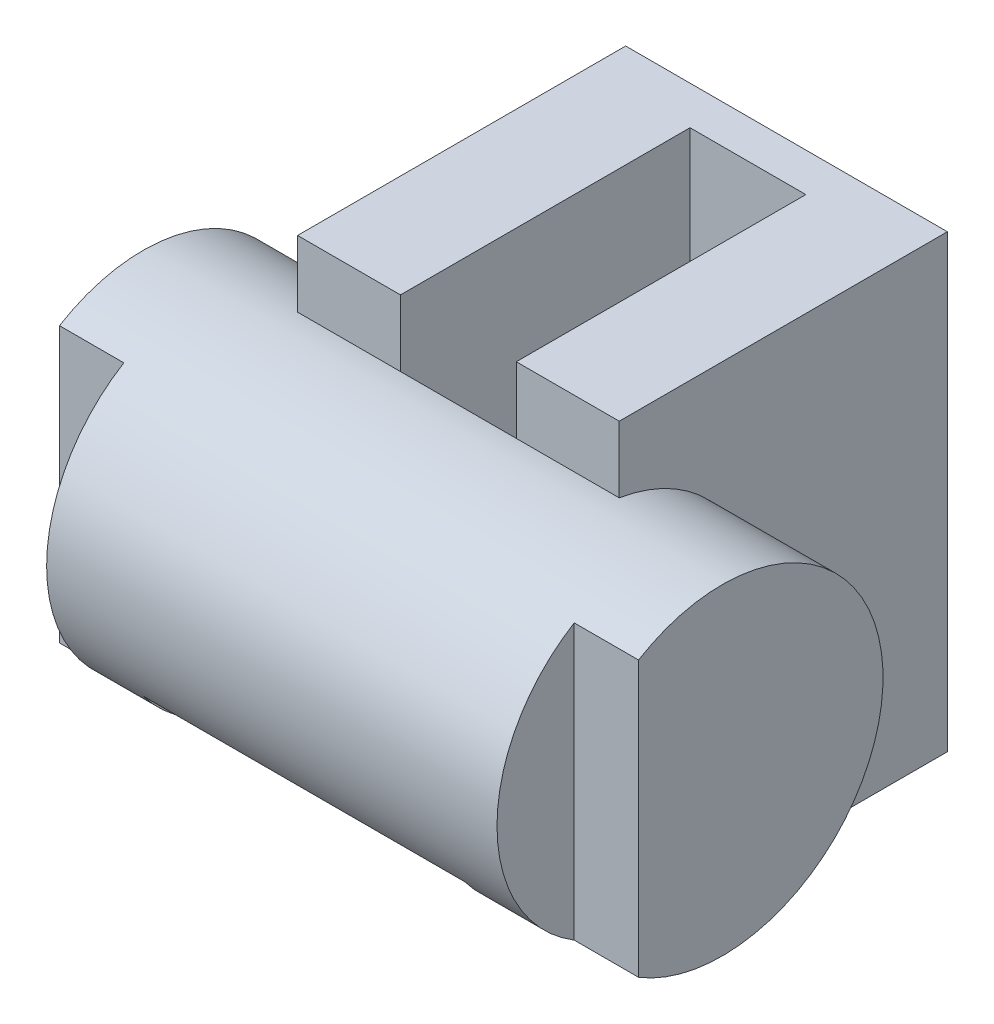
ISO-10303-21;
HEADER;
FILE_DESCRIPTION(('STEP AP214'),'2;1');
FILE_NAME('part.step','',(''),(''),'','','');
FILE_SCHEMA(('AUTOMOTIVE_DESIGN { 1 0 10303 214 1 1 1 1 }'));
ENDSEC;
DATA;
#1=APPLICATION_CONTEXT('core data for automotive mechanical design processes');
#2=APPLICATION_PROTOCOL_DEFINITION('international standard','automotive_design',2000,#1);
#3=PRODUCT_CONTEXT('',#1,'mechanical');
#4=PRODUCT('Part','Part','',(#3));
#5=PRODUCT_RELATED_PRODUCT_CATEGORY('part','',(#4));
#6=PRODUCT_DEFINITION_FORMATION('','',#4);
#7=PRODUCT_DEFINITION_CONTEXT('part definition',#1,'design');
#8=PRODUCT_DEFINITION('design','',#6,#7);
#9=PRODUCT_DEFINITION_SHAPE('','',#8);
#10=(LENGTH_UNIT() NAMED_UNIT(*) SI_UNIT(.MILLI.,.METRE.));
#11=(NAMED_UNIT(*) PLANE_ANGLE_UNIT() SI_UNIT($,.RADIAN.));
#12=(NAMED_UNIT(*) SI_UNIT($,.STERADIAN.) SOLID_ANGLE_UNIT());
#13=UNCERTAINTY_MEASURE_WITH_UNIT(LENGTH_MEASURE(1.E-05),#10,'distance_accuracy_value','');
#14=(GEOMETRIC_REPRESENTATION_CONTEXT(3) GLOBAL_UNCERTAINTY_ASSIGNED_CONTEXT((#13)) GLOBAL_UNIT_ASSIGNED_CONTEXT((#10,
#11,#12)) REPRESENTATION_CONTEXT('',''));
#15=CARTESIAN_POINT('',(0.,0.,0.));
#16=DIRECTION('',(0.,0.,1.));
#17=DIRECTION('',(1.,0.,0.));
#18=AXIS2_PLACEMENT_3D('',#15,#16,#17);
#19=CARTESIAN_POINT('',(70.,-35.,58.));
#20=DIRECTION('',(-1.,0.,0.));
#21=DIRECTION('',(0.,0.,1.));
#22=AXIS2_PLACEMENT_3D('',#19,#20,#21);
#23=CYLINDRICAL_SURFACE('',#22,25.);
#24=DIRECTION('',(-1.,0.,0.));
#25=VECTOR('',#24,1.);
#26=CARTESIAN_POINT('',(70.,-10.3220746414939,54.));
#27=LINE('',#26,#25);
#28=CARTESIAN_POINT('',(16.,-10.3220746414939,54.));
#29=VERTEX_POINT('',#28);
#30=CARTESIAN_POINT('',(34.,-10.3220746414939,54.));
#31=VERTEX_POINT('',#30);
#32=EDGE_CURVE('E214',#29,#31,#27,.F.);
#33=ORIENTED_EDGE('',*,*,#32,.F.);
#34=DIRECTION('',(-1.,0.,0.));
#35=VECTOR('',#34,1.);
#36=CARTESIAN_POINT('',(70.,-10.3220746414939,54.));
#37=LINE('',#36,#35);
#38=CARTESIAN_POINT('',(0.,-10.3220746414939,54.));
#39=VERTEX_POINT('',#38);
#40=EDGE_CURVE('E233',#29,#39,#37,.T.);
#41=ORIENTED_EDGE('',*,*,#40,.T.);
#42=CARTESIAN_POINT('',(0.,-35.,58.));
#43=DIRECTION('',(-1.,0.,0.));
#44=DIRECTION('',(0.,0.,1.));
#45=AXIS2_PLACEMENT_3D('',#42,#43,#44);
#46=CIRCLE('',#45,25.);
#47=CARTESIAN_POINT('',(0.,-50.,38.));
#48=VERTEX_POINT('',#47);
#49=EDGE_CURVE('E220',#39,#48,#46,.T.);
#50=ORIENTED_EDGE('',*,*,#49,.T.);
#51=CARTESIAN_POINT('',(0.,-35.,58.));
#52=DIRECTION('',(1.,0.,0.));
#53=DIRECTION('',(0.,0.,-1.));
#54=AXIS2_PLACEMENT_3D('',#51,#52,#53);
#55=CIRCLE('',#54,25.);
#56=CARTESIAN_POINT('',(0.,-50.,78.));
#57=VERTEX_POINT('',#56);
#58=EDGE_CURVE('E323',#48,#57,#55,.F.);
#59=ORIENTED_EDGE('',*,*,#58,.T.);
#60=DIRECTION('',(-1.,0.,0.));
#61=VECTOR('',#60,1.);
#62=CARTESIAN_POINT('',(70.,-50.,78.));
#63=LINE('',#62,#61);
#64=CARTESIAN_POINT('',(50.,-50.,78.));
#65=VERTEX_POINT('',#64);
#66=EDGE_CURVE('E52',#57,#65,#63,.F.);
#67=ORIENTED_EDGE('',*,*,#66,.T.);
#68=CARTESIAN_POINT('',(50.,-35.,58.));
#69=DIRECTION('',(-1.,0.,0.));
#70=DIRECTION('',(0.,0.,1.));
#71=AXIS2_PLACEMENT_3D('',#68,#69,#70);
#72=CIRCLE('',#71,25.);
#73=CARTESIAN_POINT('',(50.,-50.,38.));
#74=VERTEX_POINT('',#73);
#75=EDGE_CURVE('E11',#65,#74,#72,.F.);
#76=ORIENTED_EDGE('',*,*,#75,.T.);
#77=CARTESIAN_POINT('',(50.,-35.,58.));
#78=DIRECTION('',(-1.,0.,0.));
#79=DIRECTION('',(0.,0.,1.));
#80=AXIS2_PLACEMENT_3D('',#77,#78,#79);
#81=CIRCLE('',#80,25.);
#82=CARTESIAN_POINT('',(50.,-10.3220746414939,54.));
#83=VERTEX_POINT('',#82);
#84=EDGE_CURVE('E226',#83,#74,#81,.T.);
#85=ORIENTED_EDGE('',*,*,#84,.F.);
#86=DIRECTION('',(-1.,0.,0.));
#87=VECTOR('',#86,1.);
#88=CARTESIAN_POINT('',(70.,-10.3220746414939,54.));
#89=LINE('',#88,#87);
#90=EDGE_CURVE('E324',#83,#31,#89,.T.);
#91=ORIENTED_EDGE('',*,*,#90,.T.);
#92=EDGE_LOOP('',(#33,#41,#50,#59,#67,#76,#85,#91));
#93=FACE_BOUND('',#92,.T.);
#94=CARTESIAN_POINT('',(-20.,-35.,58.));
#95=DIRECTION('',(-1.,0.,0.));
#96=DIRECTION('',(0.,0.,1.));
#97=AXIS2_PLACEMENT_3D('',#94,#95,#96);
#98=CIRCLE('',#97,25.);
#99=CARTESIAN_POINT('',(-20.,-13.6458434959374,71.));
#100=VERTEX_POINT('',#99);
#101=CARTESIAN_POINT('',(-20.,-56.3541565040626,71.));
#102=VERTEX_POINT('',#101);
#103=EDGE_CURVE('E221',#100,#102,#98,.T.);
#104=ORIENTED_EDGE('',*,*,#103,.F.);
#105=DIRECTION('',(-1.,0.,0.));
#106=VECTOR('',#105,1.);
#107=CARTESIAN_POINT('',(-10.,-13.6458434959374,71.));
#108=LINE('',#107,#106);
#109=CARTESIAN_POINT('',(-10.,-13.6458434959374,71.));
#110=VERTEX_POINT('',#109);
#111=EDGE_CURVE('E69',#110,#100,#108,.T.);
#112=ORIENTED_EDGE('',*,*,#111,.F.);
#113=CARTESIAN_POINT('',(-10.,-35.,58.));
#114=DIRECTION('',(-1.,0.,0.));
#115=DIRECTION('',(0.,0.,1.));
#116=AXIS2_PLACEMENT_3D('',#113,#114,#115);
#117=CIRCLE('',#116,25.);
#118=CARTESIAN_POINT('',(-10.,-56.3541565040626,71.));
#119=VERTEX_POINT('',#118);
#120=EDGE_CURVE('E196',#119,#110,#117,.T.);
#121=ORIENTED_EDGE('',*,*,#120,.F.);
#122=DIRECTION('',(-1.,0.,0.));
#123=VECTOR('',#122,1.);
#124=CARTESIAN_POINT('',(-10.,-56.3541565040626,71.));
#125=LINE('',#124,#123);
#126=EDGE_CURVE('E198',#119,#102,#125,.T.);
#127=ORIENTED_EDGE('',*,*,#126,.T.);
#128=EDGE_LOOP('',(#104,#112,#121,#127));
#129=FACE_BOUND('',#128,.T.);
#130=CARTESIAN_POINT('',(60.,-35.,58.));
#131=DIRECTION('',(1.,0.,0.));
#132=DIRECTION('',(0.,0.,-1.));
#133=AXIS2_PLACEMENT_3D('',#130,#131,#132);
#134=CIRCLE('',#133,25.);
#135=CARTESIAN_POINT('',(60.,-13.6458434959373,71.));
#136=VERTEX_POINT('',#135);
#137=CARTESIAN_POINT('',(60.,-56.3541565040626,71.));
#138=VERTEX_POINT('',#137);
#139=EDGE_CURVE('E183',#136,#138,#134,.T.);
#140=ORIENTED_EDGE('',*,*,#139,.F.);
#141=DIRECTION('',(1.,0.,0.));
#142=VECTOR('',#141,1.);
#143=CARTESIAN_POINT('',(60.,-13.6458434959373,71.));
#144=LINE('',#143,#142);
#145=CARTESIAN_POINT('',(70.,-13.6458434959373,71.));
#146=VERTEX_POINT('',#145);
#147=EDGE_CURVE('E172',#136,#146,#144,.T.);
#148=ORIENTED_EDGE('',*,*,#147,.T.);
#149=CARTESIAN_POINT('',(70.,-35.,58.));
#150=DIRECTION('',(-1.,0.,0.));
#151=DIRECTION('',(0.,0.,1.));
#152=AXIS2_PLACEMENT_3D('',#149,#150,#151);
#153=CIRCLE('',#152,25.);
#154=CARTESIAN_POINT('',(70.,-56.3541565040626,71.));
#155=VERTEX_POINT('',#154);
#156=EDGE_CURVE('E223',#146,#155,#153,.T.);
#157=ORIENTED_EDGE('',*,*,#156,.T.);
#158=DIRECTION('',(1.,0.,0.));
#159=VECTOR('',#158,1.);
#160=CARTESIAN_POINT('',(60.,-56.3541565040626,71.));
#161=LINE('',#160,#159);
#162=EDGE_CURVE('E58',#138,#155,#161,.T.);
#163=ORIENTED_EDGE('',*,*,#162,.F.);
#164=EDGE_LOOP('',(#140,#148,#157,#163));
#165=FACE_BOUND('',#164,.T.);
#166=ADVANCED_FACE('F44',(#93,#129,#165),#23,.T.);
#167=CARTESIAN_POINT('',(70.,-35.,58.));
#168=DIRECTION('',(-1.,0.,0.));
#169=DIRECTION('',(0.,0.,1.));
#170=AXIS2_PLACEMENT_3D('',#167,#168,#169);
#171=PLANE('',#170);
#172=DIRECTION('',(0.,-1.,0.));
#173=VECTOR('',#172,1.);
#174=CARTESIAN_POINT('',(70.,0.,71.));
#175=LINE('',#174,#173);
#176=EDGE_CURVE('E177',#146,#155,#175,.T.);
#177=ORIENTED_EDGE('',*,*,#176,.T.);
#178=ORIENTED_EDGE('',*,*,#156,.F.);
#179=EDGE_LOOP('',(#177,#178));
#180=FACE_BOUND('',#179,.T.);
#181=ADVANCED_FACE('F356',(#180),#171,.F.);
#182=CARTESIAN_POINT('',(-20.,-35.,58.));
#183=DIRECTION('',(-1.,0.,0.));
#184=DIRECTION('',(0.,0.,1.));
#185=AXIS2_PLACEMENT_3D('',#182,#183,#184);
#186=PLANE('',#185);
#187=ORIENTED_EDGE('',*,*,#103,.T.);
#188=DIRECTION('',(0.,1.,0.));
#189=VECTOR('',#188,1.);
#190=CARTESIAN_POINT('',(-20.,0.,71.));
#191=LINE('',#190,#189);
#192=EDGE_CURVE('E191',#102,#100,#191,.T.);
#193=ORIENTED_EDGE('',*,*,#192,.T.);
#194=EDGE_LOOP('',(#187,#193));
#195=FACE_BOUND('',#194,.T.);
#196=ADVANCED_FACE('F361',(#195),#186,.T.);
#197=CARTESIAN_POINT('',(0.,0.,9.));
#198=DIRECTION('',(1.,0.,0.));
#199=DIRECTION('',(0.,0.,-1.));
#200=AXIS2_PLACEMENT_3D('',#197,#198,#199);
#201=PLANE('',#200);
#202=ORIENTED_EDGE('',*,*,#49,.F.);
#203=DIRECTION('',(0.,1.,0.));
#204=VECTOR('',#203,1.);
#205=CARTESIAN_POINT('',(0.,0.,54.));
#206=LINE('',#205,#204);
#207=CARTESIAN_POINT('',(0.,0.,54.));
#208=VERTEX_POINT('',#207);
#209=EDGE_CURVE('E281',#39,#208,#206,.T.);
#210=ORIENTED_EDGE('',*,*,#209,.T.);
#211=DIRECTION('',(0.,0.,-1.));
#212=VECTOR('',#211,1.);
#213=CARTESIAN_POINT('',(0.,0.,9.));
#214=LINE('',#213,#212);
#215=CARTESIAN_POINT('',(0.,0.,3.));
#216=VERTEX_POINT('',#215);
#217=EDGE_CURVE('E319',#208,#216,#214,.T.);
#218=ORIENTED_EDGE('',*,*,#217,.T.);
#219=DIRECTION('',(0.,1.,0.));
#220=VECTOR('',#219,1.);
#221=CARTESIAN_POINT('',(0.,0.,3.));
#222=LINE('',#221,#220);
#223=CARTESIAN_POINT('',(0.,-70.,3.));
#224=VERTEX_POINT('',#223);
#225=EDGE_CURVE('E257',#224,#216,#222,.T.);
#226=ORIENTED_EDGE('',*,*,#225,.F.);
#227=DIRECTION('',(0.,0.,-1.));
#228=VECTOR('',#227,1.);
#229=CARTESIAN_POINT('',(0.,-70.,9.));
#230=LINE('',#229,#228);
#231=CARTESIAN_POINT('',(0.,-70.,23.));
#232=VERTEX_POINT('',#231);
#233=EDGE_CURVE('E314',#232,#224,#230,.T.);
#234=ORIENTED_EDGE('',*,*,#233,.F.);
#235=DIRECTION('',(0.,-1.,0.));
#236=VECTOR('',#235,1.);
#237=CARTESIAN_POINT('',(0.,-70.,23.));
#238=LINE('',#237,#236);
#239=CARTESIAN_POINT('',(0.,-50.,23.));
#240=VERTEX_POINT('',#239);
#241=EDGE_CURVE('E246',#240,#232,#238,.T.);
#242=ORIENTED_EDGE('',*,*,#241,.F.);
#243=DIRECTION('',(0.,0.,1.));
#244=VECTOR('',#243,1.);
#245=CARTESIAN_POINT('',(0.,-50.,54.));
#246=LINE('',#245,#244);
#247=EDGE_CURVE('E276',#240,#48,#246,.T.);
#248=ORIENTED_EDGE('',*,*,#247,.T.);
#249=EDGE_LOOP('',(#202,#210,#218,#226,#234,#242,#248));
#250=FACE_BOUND('',#249,.T.);
#251=ADVANCED_FACE('F383',(#250),#201,.F.);
#252=CARTESIAN_POINT('',(16.,-50.,54.));
#253=DIRECTION('',(0.,-1.,0.));
#254=DIRECTION('',(0.,0.,-1.));
#255=AXIS2_PLACEMENT_3D('',#252,#253,#254);
#256=PLANE('',#255);
#257=DIRECTION('',(-1.,0.,0.));
#258=VECTOR('',#257,1.);
#259=CARTESIAN_POINT('',(16.,-50.,54.));
#260=LINE('',#259,#258);
#261=CARTESIAN_POINT('',(34.,-50.,54.));
#262=VERTEX_POINT('',#261);
#263=CARTESIAN_POINT('',(16.,-50.,54.));
#264=VERTEX_POINT('',#263);
#265=EDGE_CURVE('E202',#262,#264,#260,.T.);
#266=ORIENTED_EDGE('',*,*,#265,.F.);
#267=DIRECTION('',(0.,0.,-1.));
#268=VECTOR('',#267,1.);
#269=CARTESIAN_POINT('',(34.,-50.,54.));
#270=LINE('',#269,#268);
#271=CARTESIAN_POINT('',(34.,-50.,23.));
#272=VERTEX_POINT('',#271);
#273=EDGE_CURVE('E269',#262,#272,#270,.T.);
#274=ORIENTED_EDGE('',*,*,#273,.T.);
#275=DIRECTION('',(-1.,0.,0.));
#276=VECTOR('',#275,1.);
#277=CARTESIAN_POINT('',(34.,-50.,23.));
#278=LINE('',#277,#276);
#279=CARTESIAN_POINT('',(50.,-50.,23.));
#280=VERTEX_POINT('',#279);
#281=EDGE_CURVE('E243',#280,#272,#278,.T.);
#282=ORIENTED_EDGE('',*,*,#281,.F.);
#283=DIRECTION('',(0.,0.,-1.));
#284=VECTOR('',#283,1.);
#285=CARTESIAN_POINT('',(50.,-50.,54.));
#286=LINE('',#285,#284);
#287=EDGE_CURVE('E268',#74,#280,#286,.T.);
#288=ORIENTED_EDGE('',*,*,#287,.F.);
#289=DIRECTION('',(0.,0.,-1.));
#290=VECTOR('',#289,1.);
#291=CARTESIAN_POINT('',(50.,-50.,83.));
#292=LINE('',#291,#290);
#293=EDGE_CURVE('E219',#65,#74,#292,.T.);
#294=ORIENTED_EDGE('',*,*,#293,.F.);
#295=ORIENTED_EDGE('',*,*,#66,.F.);
#296=DIRECTION('',(0.,0.,-1.));
#297=VECTOR('',#296,1.);
#298=CARTESIAN_POINT('',(0.,-50.,83.));
#299=LINE('',#298,#297);
#300=EDGE_CURVE('E212',#57,#48,#299,.T.);
#301=ORIENTED_EDGE('',*,*,#300,.T.);
#302=ORIENTED_EDGE('',*,*,#247,.F.);
#303=DIRECTION('',(-1.,0.,0.));
#304=VECTOR('',#303,1.);
#305=CARTESIAN_POINT('',(0.,-50.,23.));
#306=LINE('',#305,#304);
#307=CARTESIAN_POINT('',(16.,-50.,23.));
#308=VERTEX_POINT('',#307);
#309=EDGE_CURVE('E251',#308,#240,#306,.T.);
#310=ORIENTED_EDGE('',*,*,#309,.F.);
#311=DIRECTION('',(0.,0.,1.));
#312=VECTOR('',#311,1.);
#313=CARTESIAN_POINT('',(16.,-50.,54.));
#314=LINE('',#313,#312);
#315=EDGE_CURVE('E280',#308,#264,#314,.T.);
#316=ORIENTED_EDGE('',*,*,#315,.T.);
#317=EDGE_LOOP('',(#266,#274,#282,#288,#294,#295,#301,#302,#310,#316));
#318=FACE_BOUND('',#317,.T.);
#319=ADVANCED_FACE('F335',(#318),#256,.T.);
#320=CARTESIAN_POINT('',(50.,0.,9.));
#321=DIRECTION('',(0.,-1.,0.));
#322=DIRECTION('',(0.,0.,-1.));
#323=AXIS2_PLACEMENT_3D('',#320,#321,#322);
#324=PLANE('',#323);
#325=DIRECTION('',(1.,0.,0.));
#326=VECTOR('',#325,1.);
#327=CARTESIAN_POINT('',(50.,0.,3.));
#328=LINE('',#327,#326);
#329=CARTESIAN_POINT('',(50.,0.,3.));
#330=VERTEX_POINT('',#329);
#331=EDGE_CURVE('E262',#216,#330,#328,.T.);
#332=ORIENTED_EDGE('',*,*,#331,.F.);
#333=ORIENTED_EDGE('',*,*,#217,.F.);
#334=DIRECTION('',(-1.,0.,0.));
#335=VECTOR('',#334,1.);
#336=CARTESIAN_POINT('',(16.,0.,54.));
#337=LINE('',#336,#335);
#338=CARTESIAN_POINT('',(16.,0.,54.));
#339=VERTEX_POINT('',#338);
#340=EDGE_CURVE('E283',#339,#208,#337,.T.);
#341=ORIENTED_EDGE('',*,*,#340,.F.);
#342=DIRECTION('',(0.,0.,1.));
#343=VECTOR('',#342,1.);
#344=CARTESIAN_POINT('',(16.,0.,20.));
#345=LINE('',#344,#343);
#346=CARTESIAN_POINT('',(16.,0.,9.));
#347=VERTEX_POINT('',#346);
#348=EDGE_CURVE('E299',#347,#339,#345,.T.);
#349=ORIENTED_EDGE('',*,*,#348,.F.);
#350=DIRECTION('',(-1.,0.,0.));
#351=VECTOR('',#350,1.);
#352=CARTESIAN_POINT('',(50.,0.,9.));
#353=LINE('',#352,#351);
#354=CARTESIAN_POINT('',(34.,0.,9.));
#355=VERTEX_POINT('',#354);
#356=EDGE_CURVE('E304',#355,#347,#353,.T.);
#357=ORIENTED_EDGE('',*,*,#356,.F.);
#358=DIRECTION('',(0.,0.,-1.));
#359=VECTOR('',#358,1.);
#360=CARTESIAN_POINT('',(34.,0.,20.));
#361=LINE('',#360,#359);
#362=CARTESIAN_POINT('',(34.,0.,54.));
#363=VERTEX_POINT('',#362);
#364=EDGE_CURVE('E293',#363,#355,#361,.T.);
#365=ORIENTED_EDGE('',*,*,#364,.F.);
#366=DIRECTION('',(1.,0.,0.));
#367=VECTOR('',#366,1.);
#368=CARTESIAN_POINT('',(34.,0.,54.));
#369=LINE('',#368,#367);
#370=CARTESIAN_POINT('',(50.,0.,54.));
#371=VERTEX_POINT('',#370);
#372=EDGE_CURVE('E272',#363,#371,#369,.T.);
#373=ORIENTED_EDGE('',*,*,#372,.T.);
#374=DIRECTION('',(0.,0.,-1.));
#375=VECTOR('',#374,1.);
#376=CARTESIAN_POINT('',(50.,0.,9.));
#377=LINE('',#376,#375);
#378=EDGE_CURVE('E307',#371,#330,#377,.T.);
#379=ORIENTED_EDGE('',*,*,#378,.T.);
#380=EDGE_LOOP('',(#332,#333,#341,#349,#357,#365,#373,#379));
#381=FACE_BOUND('',#380,.T.);
#382=ADVANCED_FACE('F50',(#381),#324,.F.);
#383=CARTESIAN_POINT('',(0.,-70.,9.));
#384=DIRECTION('',(0.,1.,0.));
#385=DIRECTION('',(0.,0.,1.));
#386=AXIS2_PLACEMENT_3D('',#383,#384,#385);
#387=PLANE('',#386);
#388=DIRECTION('',(-1.,0.,0.));
#389=VECTOR('',#388,1.);
#390=CARTESIAN_POINT('',(50.,-70.,3.));
#391=LINE('',#390,#389);
#392=CARTESIAN_POINT('',(50.,-70.,3.));
#393=VERTEX_POINT('',#392);
#394=EDGE_CURVE('E260',#393,#224,#391,.T.);
#395=ORIENTED_EDGE('',*,*,#394,.F.);
#396=DIRECTION('',(0.,0.,-1.));
#397=VECTOR('',#396,1.);
#398=CARTESIAN_POINT('',(50.,-70.,9.));
#399=LINE('',#398,#397);
#400=CARTESIAN_POINT('',(50.,-70.,23.));
#401=VERTEX_POINT('',#400);
#402=EDGE_CURVE('E315',#401,#393,#399,.T.);
#403=ORIENTED_EDGE('',*,*,#402,.F.);
#404=DIRECTION('',(1.,0.,0.));
#405=VECTOR('',#404,1.);
#406=CARTESIAN_POINT('',(50.,-70.,23.));
#407=LINE('',#406,#405);
#408=CARTESIAN_POINT('',(34.,-70.,23.));
#409=VERTEX_POINT('',#408);
#410=EDGE_CURVE('E240',#409,#401,#407,.T.);
#411=ORIENTED_EDGE('',*,*,#410,.F.);
#412=DIRECTION('',(0.,0.,-1.));
#413=VECTOR('',#412,1.);
#414=CARTESIAN_POINT('',(34.,-70.,20.));
#415=LINE('',#414,#413);
#416=CARTESIAN_POINT('',(34.,-70.,9.));
#417=VERTEX_POINT('',#416);
#418=EDGE_CURVE('E290',#409,#417,#415,.T.);
#419=ORIENTED_EDGE('',*,*,#418,.T.);
#420=DIRECTION('',(1.,0.,0.));
#421=VECTOR('',#420,1.);
#422=CARTESIAN_POINT('',(0.,-70.,9.));
#423=LINE('',#422,#421);
#424=CARTESIAN_POINT('',(16.,-70.,9.));
#425=VERTEX_POINT('',#424);
#426=EDGE_CURVE('E310',#425,#417,#423,.T.);
#427=ORIENTED_EDGE('',*,*,#426,.F.);
#428=DIRECTION('',(0.,0.,1.));
#429=VECTOR('',#428,1.);
#430=CARTESIAN_POINT('',(16.,-70.,20.));
#431=LINE('',#430,#429);
#432=CARTESIAN_POINT('',(16.,-70.,23.));
#433=VERTEX_POINT('',#432);
#434=EDGE_CURVE('E296',#425,#433,#431,.T.);
#435=ORIENTED_EDGE('',*,*,#434,.T.);
#436=DIRECTION('',(1.,0.,0.));
#437=VECTOR('',#436,1.);
#438=CARTESIAN_POINT('',(16.,-70.,23.));
#439=LINE('',#438,#437);
#440=EDGE_CURVE('E248',#232,#433,#439,.T.);
#441=ORIENTED_EDGE('',*,*,#440,.F.);
#442=ORIENTED_EDGE('',*,*,#233,.T.);
#443=EDGE_LOOP('',(#395,#403,#411,#419,#427,#435,#441,#442));
#444=FACE_BOUND('',#443,.T.);
#445=ADVANCED_FACE('F398',(#444),#387,.F.);
#446=CARTESIAN_POINT('',(50.,-70.,9.));
#447=DIRECTION('',(-1.,0.,0.));
#448=DIRECTION('',(0.,0.,1.));
#449=AXIS2_PLACEMENT_3D('',#446,#447,#448);
#450=PLANE('',#449);
#451=DIRECTION('',(0.,-1.,0.));
#452=VECTOR('',#451,1.);
#453=CARTESIAN_POINT('',(50.,0.,54.));
#454=LINE('',#453,#452);
#455=EDGE_CURVE('E263',#371,#83,#454,.T.);
#456=ORIENTED_EDGE('',*,*,#455,.T.);
#457=ORIENTED_EDGE('',*,*,#84,.T.);
#458=ORIENTED_EDGE('',*,*,#287,.T.);
#459=DIRECTION('',(0.,1.,0.));
#460=VECTOR('',#459,1.);
#461=CARTESIAN_POINT('',(50.,-50.,23.));
#462=LINE('',#461,#460);
#463=EDGE_CURVE('E239',#401,#280,#462,.T.);
#464=ORIENTED_EDGE('',*,*,#463,.F.);
#465=ORIENTED_EDGE('',*,*,#402,.T.);
#466=DIRECTION('',(0.,-1.,0.));
#467=VECTOR('',#466,1.);
#468=CARTESIAN_POINT('',(50.,0.,3.));
#469=LINE('',#468,#467);
#470=EDGE_CURVE('E259',#330,#393,#469,.T.);
#471=ORIENTED_EDGE('',*,*,#470,.F.);
#472=ORIENTED_EDGE('',*,*,#378,.F.);
#473=EDGE_LOOP('',(#456,#457,#458,#464,#465,#471,#472));
#474=FACE_BOUND('',#473,.T.);
#475=ADVANCED_FACE('F396',(#474),#450,.F.);
#476=CARTESIAN_POINT('',(0.,0.,9.));
#477=DIRECTION('',(0.,0.,1.));
#478=DIRECTION('',(1.,0.,0.));
#479=AXIS2_PLACEMENT_3D('',#476,#477,#478);
#480=PLANE('',#479);
#481=DIRECTION('',(0.,-1.,0.));
#482=VECTOR('',#481,1.);
#483=CARTESIAN_POINT('',(34.,0.,9.));
#484=LINE('',#483,#482);
#485=EDGE_CURVE('E291',#355,#417,#484,.T.);
#486=ORIENTED_EDGE('',*,*,#485,.F.);
#487=ORIENTED_EDGE('',*,*,#356,.T.);
#488=DIRECTION('',(0.,-1.,0.));
#489=VECTOR('',#488,1.);
#490=CARTESIAN_POINT('',(16.,0.,9.));
#491=LINE('',#490,#489);
#492=EDGE_CURVE('E301',#347,#425,#491,.T.);
#493=ORIENTED_EDGE('',*,*,#492,.T.);
#494=ORIENTED_EDGE('',*,*,#426,.T.);
#495=EDGE_LOOP('',(#486,#487,#493,#494));
#496=FACE_BOUND('',#495,.T.);
#497=ADVANCED_FACE('F392',(#496),#480,.T.);
#498=CARTESIAN_POINT('',(16.,0.,20.));
#499=DIRECTION('',(1.,0.,0.));
#500=DIRECTION('',(0.,0.,-1.));
#501=AXIS2_PLACEMENT_3D('',#498,#499,#500);
#502=PLANE('',#501);
#503=DIRECTION('',(0.,1.,0.));
#504=VECTOR('',#503,1.);
#505=CARTESIAN_POINT('',(16.,0.,54.));
#506=LINE('',#505,#504);
#507=EDGE_CURVE('E277',#29,#339,#506,.T.);
#508=ORIENTED_EDGE('',*,*,#507,.F.);
#509=DIRECTION('',(0.,-1.,0.));
#510=VECTOR('',#509,1.);
#511=CARTESIAN_POINT('',(16.,0.,54.));
#512=LINE('',#511,#510);
#513=EDGE_CURVE('E210',#29,#264,#512,.T.);
#514=ORIENTED_EDGE('',*,*,#513,.T.);
#515=ORIENTED_EDGE('',*,*,#315,.F.);
#516=DIRECTION('',(0.,1.,0.));
#517=VECTOR('',#516,1.);
#518=CARTESIAN_POINT('',(16.,-50.,23.));
#519=LINE('',#518,#517);
#520=EDGE_CURVE('E255',#433,#308,#519,.T.);
#521=ORIENTED_EDGE('',*,*,#520,.F.);
#522=ORIENTED_EDGE('',*,*,#434,.F.);
#523=ORIENTED_EDGE('',*,*,#492,.F.);
#524=ORIENTED_EDGE('',*,*,#348,.T.);
#525=EDGE_LOOP('',(#508,#514,#515,#521,#522,#523,#524));
#526=FACE_BOUND('',#525,.T.);
#527=ADVANCED_FACE('F390',(#526),#502,.T.);
#528=CARTESIAN_POINT('',(34.,0.,20.));
#529=DIRECTION('',(-1.,0.,0.));
#530=DIRECTION('',(0.,0.,1.));
#531=AXIS2_PLACEMENT_3D('',#528,#529,#530);
#532=PLANE('',#531);
#533=ORIENTED_EDGE('',*,*,#273,.F.);
#534=DIRECTION('',(0.,-1.,0.));
#535=VECTOR('',#534,1.);
#536=CARTESIAN_POINT('',(34.,0.,54.));
#537=LINE('',#536,#535);
#538=EDGE_CURVE('E206',#31,#262,#537,.T.);
#539=ORIENTED_EDGE('',*,*,#538,.F.);
#540=DIRECTION('',(0.,-1.,0.));
#541=VECTOR('',#540,1.);
#542=CARTESIAN_POINT('',(34.,0.,54.));
#543=LINE('',#542,#541);
#544=EDGE_CURVE('E265',#363,#31,#543,.T.);
#545=ORIENTED_EDGE('',*,*,#544,.F.);
#546=ORIENTED_EDGE('',*,*,#364,.T.);
#547=ORIENTED_EDGE('',*,*,#485,.T.);
#548=ORIENTED_EDGE('',*,*,#418,.F.);
#549=DIRECTION('',(0.,-1.,0.));
#550=VECTOR('',#549,1.);
#551=CARTESIAN_POINT('',(34.,-70.,23.));
#552=LINE('',#551,#550);
#553=EDGE_CURVE('E234',#272,#409,#552,.T.);
#554=ORIENTED_EDGE('',*,*,#553,.F.);
#555=EDGE_LOOP('',(#533,#539,#545,#546,#547,#548,#554));
#556=FACE_BOUND('',#555,.T.);
#557=ADVANCED_FACE('F382',(#556),#532,.T.);
#558=CARTESIAN_POINT('',(16.,0.,54.));
#559=DIRECTION('',(0.,0.,1.));
#560=DIRECTION('',(1.,0.,0.));
#561=AXIS2_PLACEMENT_3D('',#558,#559,#560);
#562=PLANE('',#561);
#563=ORIENTED_EDGE('',*,*,#40,.F.);
#564=ORIENTED_EDGE('',*,*,#507,.T.);
#565=ORIENTED_EDGE('',*,*,#340,.T.);
#566=ORIENTED_EDGE('',*,*,#209,.F.);
#567=EDGE_LOOP('',(#563,#564,#565,#566));
#568=FACE_BOUND('',#567,.T.);
#569=ADVANCED_FACE('F380',(#568),#562,.T.);
#570=CARTESIAN_POINT('',(34.,0.,54.));
#571=DIRECTION('',(0.,0.,1.));
#572=DIRECTION('',(1.,0.,0.));
#573=AXIS2_PLACEMENT_3D('',#570,#571,#572);
#574=PLANE('',#573);
#575=ORIENTED_EDGE('',*,*,#90,.F.);
#576=ORIENTED_EDGE('',*,*,#455,.F.);
#577=ORIENTED_EDGE('',*,*,#372,.F.);
#578=ORIENTED_EDGE('',*,*,#544,.T.);
#579=EDGE_LOOP('',(#575,#576,#577,#578));
#580=FACE_BOUND('',#579,.T.);
#581=ADVANCED_FACE('F373',(#580),#574,.T.);
#582=CARTESIAN_POINT('',(0.,0.,3.));
#583=DIRECTION('',(0.,0.,-1.));
#584=DIRECTION('',(-1.,0.,0.));
#585=AXIS2_PLACEMENT_3D('',#582,#583,#584);
#586=PLANE('',#585);
#587=ORIENTED_EDGE('',*,*,#470,.T.);
#588=ORIENTED_EDGE('',*,*,#394,.T.);
#589=ORIENTED_EDGE('',*,*,#225,.T.);
#590=ORIENTED_EDGE('',*,*,#331,.T.);
#591=EDGE_LOOP('',(#587,#588,#589,#590));
#592=FACE_BOUND('',#591,.T.);
#593=ADVANCED_FACE('F367',(#592),#586,.T.);
#594=CARTESIAN_POINT('',(0.,0.,23.));
#595=DIRECTION('',(0.,0.,-1.));
#596=DIRECTION('',(-1.,0.,0.));
#597=AXIS2_PLACEMENT_3D('',#594,#595,#596);
#598=PLANE('',#597);
#599=ORIENTED_EDGE('',*,*,#241,.T.);
#600=ORIENTED_EDGE('',*,*,#440,.T.);
#601=ORIENTED_EDGE('',*,*,#520,.T.);
#602=ORIENTED_EDGE('',*,*,#309,.T.);
#603=EDGE_LOOP('',(#599,#600,#601,#602));
#604=FACE_BOUND('',#603,.T.);
#605=ADVANCED_FACE('F354',(#604),#598,.F.);
#606=CARTESIAN_POINT('',(0.,0.,23.));
#607=DIRECTION('',(0.,0.,-1.));
#608=DIRECTION('',(-1.,0.,0.));
#609=AXIS2_PLACEMENT_3D('',#606,#607,#608);
#610=PLANE('',#609);
#611=ORIENTED_EDGE('',*,*,#553,.T.);
#612=ORIENTED_EDGE('',*,*,#410,.T.);
#613=ORIENTED_EDGE('',*,*,#463,.T.);
#614=ORIENTED_EDGE('',*,*,#281,.T.);
#615=EDGE_LOOP('',(#611,#612,#613,#614));
#616=FACE_BOUND('',#615,.T.);
#617=ADVANCED_FACE('F345',(#616),#610,.F.);
#618=CARTESIAN_POINT('',(50.,-70.,83.));
#619=DIRECTION('',(-1.,0.,0.));
#620=DIRECTION('',(0.,0.,1.));
#621=AXIS2_PLACEMENT_3D('',#618,#619,#620);
#622=PLANE('',#621);
#623=ORIENTED_EDGE('',*,*,#293,.T.);
#624=ORIENTED_EDGE('',*,*,#75,.F.);
#625=EDGE_LOOP('',(#623,#624));
#626=FACE_BOUND('',#625,.T.);
#627=ADVANCED_FACE('F338',(#626),#622,.T.);
#628=CARTESIAN_POINT('',(0.,-50.,83.));
#629=DIRECTION('',(1.,0.,0.));
#630=DIRECTION('',(0.,0.,-1.));
#631=AXIS2_PLACEMENT_3D('',#628,#629,#630);
#632=PLANE('',#631);
#633=ORIENTED_EDGE('',*,*,#300,.F.);
#634=ORIENTED_EDGE('',*,*,#58,.F.);
#635=EDGE_LOOP('',(#633,#634));
#636=FACE_BOUND('',#635,.T.);
#637=ADVANCED_FACE('F341',(#636),#632,.T.);
#638=CARTESIAN_POINT('',(16.,0.,54.));
#639=DIRECTION('',(0.,0.,1.));
#640=DIRECTION('',(1.,0.,0.));
#641=AXIS2_PLACEMENT_3D('',#638,#639,#640);
#642=PLANE('',#641);
#643=ORIENTED_EDGE('',*,*,#32,.T.);
#644=ORIENTED_EDGE('',*,*,#538,.T.);
#645=ORIENTED_EDGE('',*,*,#265,.T.);
#646=ORIENTED_EDGE('',*,*,#513,.F.);
#647=EDGE_LOOP('',(#643,#644,#645,#646));
#648=FACE_BOUND('',#647,.T.);
#649=ADVANCED_FACE('F348',(#648),#642,.F.);
#650=CARTESIAN_POINT('',(-10.,0.,71.));
#651=DIRECTION('',(0.,0.,1.));
#652=DIRECTION('',(1.,0.,0.));
#653=AXIS2_PLACEMENT_3D('',#650,#651,#652);
#654=PLANE('',#653);
#655=ORIENTED_EDGE('',*,*,#192,.F.);
#656=ORIENTED_EDGE('',*,*,#126,.F.);
#657=DIRECTION('',(0.,1.,0.));
#658=VECTOR('',#657,1.);
#659=CARTESIAN_POINT('',(-10.,0.,71.));
#660=LINE('',#659,#658);
#661=EDGE_CURVE('E193',#119,#110,#660,.T.);
#662=ORIENTED_EDGE('',*,*,#661,.T.);
#663=ORIENTED_EDGE('',*,*,#111,.T.);
#664=EDGE_LOOP('',(#655,#656,#662,#663));
#665=FACE_BOUND('',#664,.T.);
#666=ADVANCED_FACE('F438',(#665),#654,.T.);
#667=CARTESIAN_POINT('',(-10.,0.,0.));
#668=DIRECTION('',(-1.,0.,0.));
#669=DIRECTION('',(0.,0.,1.));
#670=AXIS2_PLACEMENT_3D('',#667,#668,#669);
#671=PLANE('',#670);
#672=ORIENTED_EDGE('',*,*,#661,.F.);
#673=ORIENTED_EDGE('',*,*,#120,.T.);
#674=EDGE_LOOP('',(#672,#673));
#675=FACE_BOUND('',#674,.T.);
#676=ADVANCED_FACE('F443',(#675),#671,.T.);
#677=CARTESIAN_POINT('',(60.,0.,71.));
#678=DIRECTION('',(0.,0.,1.));
#679=DIRECTION('',(1.,0.,0.));
#680=AXIS2_PLACEMENT_3D('',#677,#678,#679);
#681=PLANE('',#680);
#682=ORIENTED_EDGE('',*,*,#176,.F.);
#683=ORIENTED_EDGE('',*,*,#147,.F.);
#684=DIRECTION('',(0.,-1.,0.));
#685=VECTOR('',#684,1.);
#686=CARTESIAN_POINT('',(60.,0.,71.));
#687=LINE('',#686,#685);
#688=EDGE_CURVE('E180',#136,#138,#687,.T.);
#689=ORIENTED_EDGE('',*,*,#688,.T.);
#690=ORIENTED_EDGE('',*,*,#162,.T.);
#691=EDGE_LOOP('',(#682,#683,#689,#690));
#692=FACE_BOUND('',#691,.T.);
#693=ADVANCED_FACE('F176',(#692),#681,.T.);
#694=CARTESIAN_POINT('',(60.,0.,0.));
#695=DIRECTION('',(1.,0.,0.));
#696=DIRECTION('',(0.,0.,-1.));
#697=AXIS2_PLACEMENT_3D('',#694,#695,#696);
#698=PLANE('',#697);
#699=ORIENTED_EDGE('',*,*,#688,.F.);
#700=ORIENTED_EDGE('',*,*,#139,.T.);
#701=EDGE_LOOP('',(#699,#700));
#702=FACE_BOUND('',#701,.T.);
#703=ADVANCED_FACE('F190',(#702),#698,.T.);
#704=CLOSED_SHELL('',(#166,#181,#196,#251,#319,#382,#445,#475,#497,#527,#557,#569,#581,#593,
#605,#617,#627,#637,#649,#666,#676,#693,#703));
#705=MANIFOLD_SOLID_BREP('B2',#704);
#706=ADVANCED_BREP_SHAPE_REPRESENTATION('',(#18,#705),#14);
#707=SHAPE_DEFINITION_REPRESENTATION(#9,#706);
ENDSEC;
END-ISO-10303-21;
